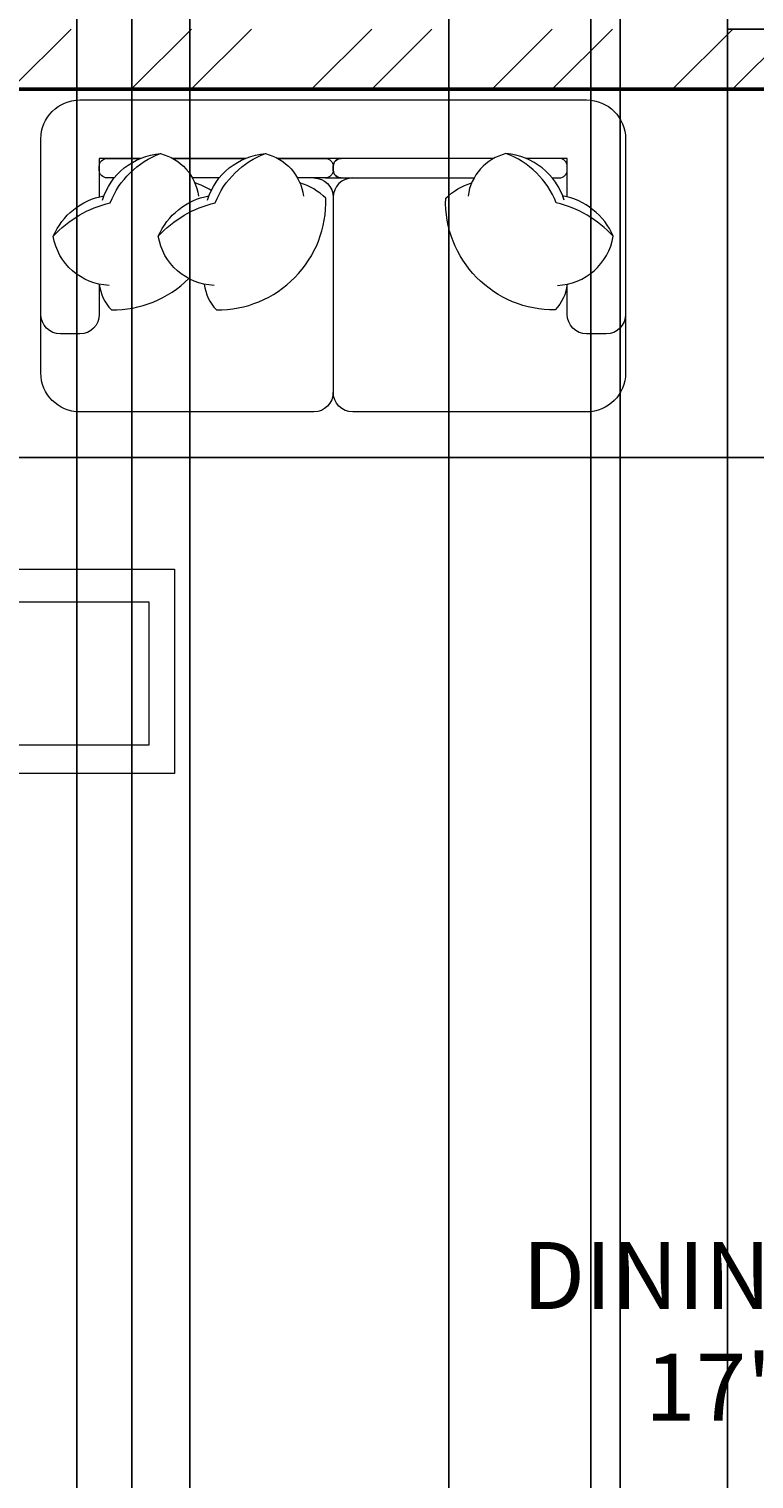
# Model space of a CAD drawing. Units: inches. Extents: x 2310 to 2937, y 1113 to 2410.
# Tile 6 of 23: x 2472 to 2526, y 1891 to 2000. Entities that reach past the tile are written whole.
import ezdxf

# ---------------------------------------------------------------- set-up
doc = ezdxf.new("R2010")
doc.units = ezdxf.units.IN
for name, color, linetype, lineweight in [('A-ANNO-DIMS', 2, 'Continuous', 18), ('A-AREA-IDEN', 7, 'Continuous', 18), ('A-FURN', 8, 'Continuous', 18), ('A-WALL', 7, 'Continuous', 50), ('A-WALL-PATT', 85, 'Continuous', 13)]:
    doc.layers.add(name, color=color, linetype=linetype, lineweight=lineweight)
doc.styles.get("Standard").update_dxf_attribs({"font": 'arial.ttf'})
doc.dimstyles.get("Standard").update_dxf_attribs({"dimtxt": 0.18, "dimasz": 0.18, "dimexe": 0.18, "dimexo": 0.0625, "dimgap": 0.09, "dimtad": 0, "dimtih": 1, "dimtoh": 1, "dimdec": 4, "dimzin": 0, "dimdsep": 46, "dimtxsty": 'Standard', "dimcen": 0.09, "dimadec": 0, "dimazin": 0, "dimtfac": 1, "dimtdec": 4, "dimtofl": 0, "dimtmove": 0, "dimatfit": 3, "dimfxl": 1, "dimtolj": 1, "dimtzin": 0, "dimarcsym": 0})

# ---------------------------------------------------------------- blocks, each defined once
blk = doc.blocks.new('*D41')
at = {"layer": 'A-ANNO-DIMS', "color": 0, "lineweight": -2, "transparency": 16777216}
for p, q in [((2479.99, 2347.45), (2479.99, 1649.5)), ((2503.66, 2347.45), (2503.66, 1649.5)), ((2480.17, 1649.68), (2491.36, 1649.68)), ((2503.48, 1649.68), (2492.29, 1649.68))]:
    blk.add_line(p, q, dxfattribs=at)
at = {"layer": 'A-ANNO-DIMS', "color": 0, "transparency": 16777216}
for points in [[(2480.17, 1649.71), (2480.17, 1649.65), (2479.99, 1649.68)], [(2503.48, 1649.71), (2503.48, 1649.65), (2503.66, 1649.68)]]:
    blk.add_solid(points, dxfattribs=at)
at = {"layer": 'Defpoints', "color": 0, "transparency": 16777216}
for p in [(2479.99, 2347.51), (2503.66, 2347.51), (2503.66, 1649.68)]:
    blk.add_point(p, dxfattribs=at)
at = {"layer": 'A-ANNO-DIMS', "color": 0, "transparency": 16777216, "insert": (2491.82, 1649.68), "char_height": 0.18, "attachment_point": 5}
blk.add_mtext('\\A1;23.676', dxfattribs=at)
blk = doc.blocks.new('*D57')
at = {"layer": 'A-ANNO-DIMS', "color": 0, "lineweight": -2, "transparency": 16777216}
for p, q in [((2403.55, 1995.01), (2858.02, 1995.01)), ((2857.84, 1994.83), (2857.84, 1981.45)), ((2857.84, 1967.7), (2857.84, 1981.09)), ((2403.55, 1967.52), (2858.02, 1967.52))]:
    blk.add_line(p, q, dxfattribs=at)
at = {"layer": 'A-ANNO-DIMS', "color": 0, "transparency": 16777216}
for points in [[(2857.81, 1994.83), (2857.87, 1994.83), (2857.84, 1995.01)], [(2857.81, 1967.7), (2857.87, 1967.7), (2857.84, 1967.52)]]:
    blk.add_solid(points, dxfattribs=at)
at = {"layer": 'Defpoints', "color": 0, "transparency": 16777216}
for p in [(2403.49, 1995.01), (2403.49, 1967.52), (2857.84, 1967.52)]:
    blk.add_point(p, dxfattribs=at)
at = {"layer": 'A-ANNO-DIMS', "color": 0, "transparency": 16777216, "insert": (2857.84, 1981.27), "char_height": 0.18, "attachment_point": 5}
blk.add_mtext('\\A1;27.49', dxfattribs=at)
blk = doc.blocks.new('*D61')
at = {"layer": 'A-ANNO-DIMS', "color": 0, "lineweight": -2, "transparency": 16777216}
for p, q in [((2484.33, 2205.95), (2484.33, 1649.5)), ((2514.27, 2205.95), (2514.27, 1649.5)), ((2484.51, 1649.68), (2498.9, 1649.68)), ((2514.09, 1649.68), (2499.69, 1649.68))]:
    blk.add_line(p, q, dxfattribs=at)
at = {"layer": 'A-ANNO-DIMS', "color": 0, "transparency": 16777216}
for points in [[(2484.51, 1649.71), (2484.51, 1649.65), (2484.33, 1649.68)], [(2514.09, 1649.71), (2514.09, 1649.65), (2514.27, 1649.68)]]:
    blk.add_solid(points, dxfattribs=at)
at = {"layer": 'Defpoints', "color": 0, "transparency": 16777216}
for p in [(2484.33, 2206.01), (2514.27, 2206.01), (2514.27, 1649.68)]:
    blk.add_point(p, dxfattribs=at)
at = {"layer": 'A-ANNO-DIMS', "color": 0, "transparency": 16777216, "insert": (2499.3, 1649.68), "char_height": 0.18, "attachment_point": 5}
blk.add_mtext('\\A1;29.94', dxfattribs=at)
blk = doc.blocks.new('*D63')
at = {"layer": 'A-ANNO-DIMS', "color": 0, "lineweight": -2, "transparency": 16777216}
for p, q in [((2436.46, 1999.45), (2436.46, 1649.5)), ((2524.46, 1999.45), (2524.46, 1649.5)), ((2436.64, 1649.68), (2480.25, 1649.68)), ((2524.28, 1649.68), (2480.68, 1649.68))]:
    blk.add_line(p, q, dxfattribs=at)
at = {"layer": 'A-ANNO-DIMS', "color": 0, "transparency": 16777216}
for points in [[(2436.64, 1649.71), (2436.64, 1649.65), (2436.46, 1649.68)], [(2524.28, 1649.71), (2524.28, 1649.65), (2524.46, 1649.68)]]:
    blk.add_solid(points, dxfattribs=at)
at = {"layer": 'Defpoints', "color": 0, "transparency": 16777216}
for p in [(2436.46, 1999.51), (2524.46, 1999.51), (2524.46, 1649.68)]:
    blk.add_point(p, dxfattribs=at)
at = {"layer": 'A-ANNO-DIMS', "color": 0, "transparency": 16777216, "insert": (2480.46, 1649.68), "char_height": 0.18, "attachment_point": 5}
blk.add_mtext('\\A1;88', dxfattribs=at)
blk = doc.blocks.new('*D64')
at = {"layer": 'A-ANNO-DIMS', "color": 0, "lineweight": -2, "transparency": 16777216}
for p, q in [((2524.527191, 2046.513944), (2858.015941, 2046.513944)), ((2857.835941, 2046.333944), (2857.835941, 2023.193944)), ((2857.835941, 1999.693944), (2857.835941, 2022.833944)), ((2524.527191, 1999.513944), (2858.015941, 1999.513944))]:
    blk.add_line(p, q, dxfattribs=at)
at = {"layer": 'A-ANNO-DIMS', "color": 0, "transparency": 16777216}
for points in [[(2857.805941, 2046.333944), (2857.865941, 2046.333944), (2857.835941, 2046.513944)], [(2857.805941, 1999.693944), (2857.865941, 1999.693944), (2857.835941, 1999.513944)]]:
    blk.add_solid(points, dxfattribs=at)
at = {"layer": 'Defpoints', "color": 0, "transparency": 16777216}
for p in [(2524.464691, 2046.513944), (2857.835941, 2046.513944), (2524.464691, 1999.513944)]:
    blk.add_point(p, dxfattribs=at)
at = {"layer": 'A-ANNO-DIMS', "color": 0, "transparency": 16777216, "insert": (2857.835941, 2023.013944), "char_height": 0.18, "attachment_point": 5}
blk.add_mtext('\\A1;47', dxfattribs=at)
blk = doc.blocks.new('*D66')
at = {"layer": 'A-ANNO-DIMS', "color": 0, "lineweight": -2, "transparency": 16777216}
for p, q in [((2516.46, 2093.45), (2516.46, 1649.5)), ((2524.46, 2093.45), (2524.46, 1649.5)), ((2516.64, 1649.68), (2520.32, 1649.68)), ((2524.28, 1649.68), (2520.61, 1649.68))]:
    blk.add_line(p, q, dxfattribs=at)
at = {"layer": 'A-ANNO-DIMS', "color": 0, "transparency": 16777216}
for points in [[(2516.64, 1649.71), (2516.64, 1649.65), (2516.46, 1649.68)], [(2524.28, 1649.71), (2524.28, 1649.65), (2524.46, 1649.68)]]:
    blk.add_solid(points, dxfattribs=at)
at = {"layer": 'Defpoints', "color": 0, "transparency": 16777216}
for p in [(2516.46, 2093.51), (2524.46, 2093.51), (2524.46, 1649.68)]:
    blk.add_point(p, dxfattribs=at)
at = {"layer": 'A-ANNO-DIMS', "color": 0, "transparency": 16777216, "insert": (2520.46, 1649.68), "char_height": 0.18, "attachment_point": 5}
blk.add_mtext('\\A1;8', dxfattribs=at)
blk = doc.blocks.new('*D69')
at = {"layer": 'A-ANNO-DIMS', "color": 0, "lineweight": -2, "transparency": 16777216}
for p, q in [((2441.86, 2131.96), (2441.86, 1649.5)), ((2475.89, 2131.96), (2475.89, 1649.5)), ((2442.04, 1649.68), (2458.48, 1649.68)), ((2475.71, 1649.68), (2459.27, 1649.68))]:
    blk.add_line(p, q, dxfattribs=at)
at = {"layer": 'A-ANNO-DIMS', "color": 0, "transparency": 16777216}
for points in [[(2442.04, 1649.71), (2442.04, 1649.65), (2441.86, 1649.68)], [(2475.71, 1649.71), (2475.71, 1649.65), (2475.89, 1649.68)]]:
    blk.add_solid(points, dxfattribs=at)
at = {"layer": 'Defpoints', "color": 0, "transparency": 16777216}
for p in [(2441.86, 2132.02), (2475.89, 2132.02), (2475.89, 1649.68)]:
    blk.add_point(p, dxfattribs=at)
at = {"layer": 'A-ANNO-DIMS', "color": 0, "transparency": 16777216, "insert": (2458.88, 1649.68), "char_height": 0.18, "attachment_point": 5}
blk.add_mtext('\\A1;34.03', dxfattribs=at)

msp = doc.modelspace()

# ---------------------------------------------------------------- hatches: boundary and pattern name
at = {"layer": 'A-WALL-PATT'}
h = msp.add_hatch(dxfattribs=at)
h.set_pattern_fill('ANSI32', color=256)
h.paths.add_polyline_path([(2639.1394, 2356.5139), (2563.662, 2356.5139), (2563.662, 2347.5139), (2606.9859, 2347.5139), (2606.9859, 2210.5139), (2514.2692, 2210.5139), (2514.2692, 2206.0139), (2606.9859, 2206.0139), (2606.9859, 2098.0139), (2602.689, 2098.0139), (2602.689, 2093.5139), (2615.5262, 2093.5139), (2615.5262, 2095.7639), (2615.5262, 2098.0139), (2611.4859, 2098.0139), (2611.4859, 2206.0139), (2703.9391, 2206.0139), (2703.9391, 2208.2639), (2703.9391, 2210.5139), (2611.4859, 2210.5139), (2611.4859, 2347.5139), (2639.1394, 2347.5139)])
h.paths.add_polyline_path([(2823.9859, 2356.5139), (2699.1394, 2356.5139), (2699.1394, 2347.5139), (2738.4859, 2347.5139), (2738.4859, 2343.9266), (2742.9859, 2343.9266), (2742.9859, 2347.5139), (2814.9859, 2347.5139), (2814.9859, 2336.76), (2823.9859, 2336.76)])
h.paths.add_polyline_path([(2823.9859, 2312.76), (2814.9859, 2312.76), (2814.9859, 2299.5139), (2742.9859, 2299.5139), (2742.9859, 2323.0159), (2740.7359, 2323.0159), (2738.4859, 2323.0159), (2738.4859, 2210.5139), (2734.5483, 2210.5139), (2734.5483, 2206.0139), (2746.8769, 2206.0139), (2746.8769, 2208.2639), (2746.8769, 2210.5139), (2742.9859, 2210.5139), (2742.9859, 2295.0139), (2814.9859, 2295.0139), (2814.9859, 2269.8977), (2823.9859, 2269.8977)])
h.paths.add_polyline_path([(2823.9859, 2210.5139), (2823.9859, 2233.8977), (2819.4859, 2233.8977), (2814.9859, 2233.8977), (2814.9859, 2210.5139), (2769.9745, 2210.5139), (2769.9745, 2206.0139), (2814.9859, 2206.0139), (2814.9859, 2178.3027), (2823.9859, 2178.3027)])
h.paths.add_polyline_path([(2823.9859, 2118.3027), (2819.4859, 2118.3027), (2814.9859, 2118.3027), (2814.9859, 2098.0139), (2647.0333, 2098.0139), (2647.0333, 2093.5139), (2814.9859, 2093.5139), (2814.9859, 1999.5139), (2650.6052, 1999.5139), (2650.6052, 1995.0139), (2814.9859, 1995.0139), (2814.9859, 1969.9784), (2823.9859, 1969.9784)])
h.paths.add_polyline_path([(2403.4859, 2093.5139), (2569.9888, 2093.5139), (2569.9888, 2095.7639), (2569.9888, 2098.0139), (2403.4859, 2098.0139), (2403.4859, 2131.7587), (2394.4859, 2131.7587), (2394.4859, 1967.522), (2403.4859, 1967.522), (2403.4859, 1995.0139), (2569.8903, 1995.0139), (2569.8903, 1997.2639), (2569.8903, 1999.5139), (2403.4859, 1999.5139)])
h.paths.add_polyline_path([(2503.662, 2356.5139), (2394.4859, 2356.5139), (2394.4859, 2337.9231), (2398.9859, 2337.9231), (2403.4859, 2337.9231), (2403.4859, 2347.5139), (2475.4859, 2347.5139), (2475.4859, 2343.0384), (2479.9859, 2343.0384), (2479.9859, 2347.5139), (2503.662, 2347.5139)])
h.paths.add_polyline_path([(2498.3065, 1745.5139), (2479.9859, 1745.5139), (2479.9859, 1749.1663), (2477.7359, 1749.1663), (2475.4859, 1749.1663), (2475.4859, 1745.5139), (2403.4859, 1745.5139), (2403.4859, 1753.6409), (2398.9859, 1753.6409), (2394.4859, 1753.6409), (2394.4859, 1736.5139), (2498.3065, 1736.5139), (2498.3065, 1741.0139)])
h.paths.add_polyline_path([(2479.9859, 1882.5139), (2483.9367, 1882.5139), (2483.9367, 1887.0139), (2471.5501, 1887.0139), (2471.5501, 1885.1969), (2471.5501, 1882.5139), (2475.4859, 1882.5139), (2475.4859, 1798.0139), (2403.4859, 1798.0139), (2403.4859, 1828.0433), (2402.2852, 1828.0433), (2394.4859, 1828.0433), (2394.4859, 1777.6409), (2403.4859, 1777.6409), (2403.4859, 1793.5139), (2475.4859, 1793.5139), (2475.4859, 1769.1696), (2479.9859, 1769.1696)])
h.paths.add_polyline_path([(2403.4859, 1907.522), (2398.9859, 1907.522), (2394.4859, 1907.522), (2394.4859, 1864.0433), (2403.4859, 1864.0433), (2403.4859, 1882.5139), (2448.9325, 1882.5139), (2448.9325, 1884.7639), (2448.9325, 1887.0139), (2403.4859, 1887.0139)])
h.paths.add_polyline_path([(2702.2061, 1887.0139), (2611.4859, 1887.0139), (2611.4859, 1995.0139), (2615.6132, 1995.0139), (2615.6132, 1999.5139), (2602.4798, 1999.5139), (2602.4798, 1997.2639), (2602.4798, 1995.0139), (2606.9859, 1995.0139), (2606.9859, 1887.0139), (2516.2443, 1887.0139), (2516.2443, 1884.7639), (2516.2443, 1882.5139), (2606.9859, 1882.5139), (2606.9859, 1745.5139), (2558.3065, 1745.5139), (2558.3065, 1736.5139), (2638.8921, 1736.5139), (2638.8921, 1741.0139), (2638.8921, 1745.5139), (2611.4859, 1745.5139), (2611.4859, 1882.5139), (2702.2061, 1882.5139)])
h.paths.add_polyline_path([(2823.9859, 1909.9784), (2819.4859, 1909.9784), (2814.9859, 1909.9784), (2814.9859, 1887.0139), (2769.144, 1887.0139), (2769.144, 1884.7639), (2769.144, 1882.5139), (2814.9859, 1882.5139), (2814.9859, 1854.1704), (2823.9859, 1854.1704)])
h.paths.add_polyline_path([(2823.9859, 1818.1704), (2819.4859, 1818.1704), (2814.9859, 1818.1704), (2814.9859, 1798.0139), (2742.9859, 1798.0139), (2742.9859, 1882.5139), (2746.805, 1882.5139), (2746.805, 1887.0139), (2733.7334, 1887.0139), (2733.7334, 1884.7639), (2733.7334, 1882.5139), (2738.4859, 1882.5139), (2738.4859, 1771.1728), (2740.7359, 1771.1728), (2742.9859, 1771.1728), (2742.9859, 1793.5139), (2814.9859, 1793.5139), (2814.9859, 1783.6684), (2823.9859, 1783.6684)])
h.paths.add_polyline_path([(2823.9859, 1759.6684), (2814.9859, 1759.6684), (2814.9859, 1745.5139), (2742.9859, 1745.5139), (2742.9859, 1748.9831), (2740.7359, 1748.9831), (2738.4859, 1748.9831), (2738.4859, 1745.5139), (2698.8921, 1745.5139), (2698.8921, 1736.5139), (2823.9859, 1736.5139)])

# ---------------------------------------------------------------- linework, layer by layer
at = {"layer": 'A-FURN', "ltscale": 0.03}
msp.add_lwpolyline([(2496.4919, 1970.9338, -0.41421356), (2495.0368, 1972.389, -0.41421356), (2493.5816, 1970.9338), (2476.1193, 1970.9338, -0.41421356), (2473.2089, 1973.8442), (2473.2089, 1991.3064, -0.41421356), (2476.1193, 1994.2168), (2513.9542, 1994.2168, -0.41421356), (2516.8646, 1991.3064), (2516.8646, 1973.8442, -0.41421356), (2513.9542, 1970.9338), (2496.4919, 1970.9338, -0.41421356), (2495.0368, 1972.389, -0.41421356), (2493.5816, 1970.9338)], format="xyb", dxfattribs=at)
at = {"layer": 'A-FURN'}
for points in [[(2474.1351, 1984.0442, -0.14772988), (2478.3882, 1986.5451, -0.21334276), (2482.1409, 1990.2131, -0.17866181)], [(2480.6358, 1989.8512), (2477.5745, 1989.8512), (2477.5745, 1986.9914, -0.41421356)], [(2478.685, 1988.396), (2478.1566, 1988.396, -0.41421356), (2477.5745, 1988.9781), (2477.5745, 1989.2692, -0.41421356), (2478.1566, 1989.8512)], [(2477.8006, 1986.7444, -0.30666349), (2482.1409, 1990.2131, -0.30632997), (2484.9763, 1987.0453, 0.87284716)], [(2478.1566, 1989.8512), (2480.6358, 1989.8512, -0.41421356)], [(2481.9741, 1984.0442, -0.14772988), (2486.2272, 1986.5451, -0.21334276), (2489.9799, 1990.2131, -0.17866181)], [(2483.0567, 1989.8512), (2488.4748, 1989.8512, -0.41421356)], [(2485.6396, 1986.7444, -0.30666349), (2489.9799, 1990.2131, -0.30632997), (2492.8153, 1987.0453, 0.87284716)], [(2490.8958, 1989.8512), (2494.4547, 1989.8512, -0.41421356), (2495.0368, 1989.2692), (2495.0368, 1988.9781, -0.41421356), (2494.4547, 1988.396), (2492.361, 1988.396, -0.41421356)], [(2507.0168, 1989.8512), (2495.6188, 1989.8512, 0.41421356), (2495.0368, 1989.2692), (2495.0368, 1988.9781, 0.41421356), (2495.6188, 1988.396), (2505.5515, 1988.396, 0.41421356)], [(2512.2729, 1986.7444, 0.30666349), (2507.9326, 1990.2131, 0.30632997), (2505.0972, 1987.0453, -0.87284716)], [(2515.9385, 1984.0442, 0.14772988), (2511.6854, 1986.5451, 0.21334276), (2507.9326, 1990.2131, 0.17866181)], [(2511.9169, 1989.8512), (2509.4377, 1989.8512, 0.41421356)], [(2511.3885, 1988.396), (2511.9169, 1988.396, 0.41421356), (2512.499, 1988.9781), (2512.499, 1989.2692, 0.41421356), (2511.9169, 1989.8512)], [(2486.524, 1988.396), (2484.522, 1988.396, -0.41421356)], [(2493.5816, 1988.396, -0.41421356), (2495.0368, 1986.9409)], [(2493.5816, 1988.396, -0.41421356), (2495.0368, 1986.9409), (2495.0368, 1972.389, -0.41421356)], [(2496.4919, 1988.396, 0.41421356), (2495.0368, 1986.9409)], [(2496.4919, 1988.396, 0.41421356), (2495.0368, 1986.9409), (2495.0368, 1972.389, 0.41421356)], [(2485.9242, 1987.4587, 0.07186538), (2484.7041, 1988.0276, -7.11546429)], [(2485.4104, 1980.465, 0.16554063), (2486.3106, 1978.5423, 0.42598917), (2494.4832, 1986.8786, 0.12152332), (2492.5432, 1988.0276, -7.11546429)], [(2512.5022, 1980.465, -0.16554063), (2511.602, 1978.5423, -0.42598917), (2503.4293, 1986.8786, -0.12152332), (2505.3694, 1988.0276, 7.11546429)], [(2478.3048, 1980.3763, -0.35677236), (2474.1351, 1984.0442, -0.24954205), (2477.9132, 1987.067, 9.61688035)], [(2486.1438, 1980.3763, -0.35677236), (2481.9741, 1984.0442, -0.24954205), (2485.7522, 1987.067, 9.61688035)], [(2511.7687, 1980.3763, 0.35677236), (2515.9385, 1984.0442, 0.24954205), (2512.1603, 1987.067, -9.61688035)], [(2477.5713, 1980.465, 0.16554063), (2478.4715, 1978.5423, 0.20023115), (2484.2481, 1980.884, 0.12152332)], [(2477.5745, 1980.4643), (2477.5745, 1978.2097, -0.41421356), (2476.1193, 1976.7545), (2474.6641, 1976.7545, -0.41421356), (2473.2089, 1978.2097)], [(2516.8646, 1978.2097, -0.41421356), (2515.4094, 1976.7545), (2513.9542, 1976.7545, -0.41421356), (2512.499, 1978.2097), (2512.499, 1980.4643)]]:
    msp.add_lwpolyline(points, format="xyb", dxfattribs=at)
for points in [[(2488.4748, 1989.8512), (2483.0567, 1989.8512)], [(2507.0168, 1989.8512), (2490.8958, 1989.8512)], [(2512.499, 1986.9914), (2512.499, 1989.8512), (2509.4377, 1989.8512)]]:
    msp.add_lwpolyline(points, dxfattribs=at)
msp.add_lwpolyline([(2495.6188, 1989.8512), (2494.4547, 1989.8512, -0.41421356), (2495.0368, 1989.2692), (2495.0368, 1988.9781, -0.41421356), (2494.4547, 1988.396), (2495.6188, 1988.396, -0.41421356), (2495.0368, 1988.9781), (2495.0368, 1989.2692, -0.41421356)], format="xyb", close=True, dxfattribs=at)
for points in [[(2449.1475, 1959.1855), (2483.1791, 1959.1855), (2483.1791, 1943.9281), (2449.1475, 1943.9281)], [(2450.9745, 1956.7439), (2481.2801, 1956.7439), (2481.2801, 1946.0624), (2450.9745, 1946.0624)]]:
    msp.add_lwpolyline(points, close=True, dxfattribs=at)
at = {"layer": 'A-WALL'}
msp.add_line((2403.4859, 1995.0139), (2571.4589, 1995.0139), dxfattribs=at)

# ---------------------------------------------------------------- texts
at = {"layer": 'A-AREA-IDEN', "insert": (2495.3926, 1908.9628), "char_height": 5, "attachment_point": 1}
msp.add_mtext_dynamic_manual_height_columns("         DINING CUM LIVING\\P               17'X9'", width=186.629206, gutter_width=12.5, heights=[0], dxfattribs=at)

# ---------------------------------------------------------------- dimensions: what is measured, and where the dimension line sits
at = {"layer": 'A-ANNO-DIMS'}
for base, p1, p2, override, picture, middle in [((2503.662, 1649.6807), (2479.9859, 2347.5139), (2503.662, 2347.5139), {"dimdec": 3, "dimlfac": 1, "dimrnd": 0, "dimzin": 0, "dimdsep": 46, "dimlunit": 2}, '*D41', (2491.824, 1649.6807)), ((2514.2692, 1649.6807), (2484.3278, 2206.0139), (2514.2692, 2206.0139), {"dimdec": 2, "dimlfac": 1, "dimrnd": 0, "dimzin": 0, "dimdsep": 46, "dimlunit": 2}, '*D61', (2499.2985, 1649.6807)), ((2475.8929, 1649.6807), (2441.8613, 2132.0241), (2475.8929, 2132.0241), {"dimdec": 2, "dimlfac": 1, "dimrnd": 0, "dimzin": 0, "dimdsep": 46, "dimlunit": 2}, '*D69', (2458.8771, 1649.6807)), ((2524.4647, 1649.6807), (2516.4647, 2093.5139), (2524.4647, 2093.5139), {"dimdec": 0, "dimlfac": 1, "dimrnd": 0, "dimzin": 0, "dimdsep": 46, "dimlunit": 2}, '*D66', (2520.4647, 1649.6807)), ((2524.4647, 1649.6807), (2436.4647, 1999.5139), (2524.4647, 1999.5139), {"dimdec": 0, "dimlfac": 1, "dimrnd": 0, "dimzin": 0, "dimdsep": 46, "dimlunit": 2}, '*D63', (2480.4647, 1649.6807))]:
    dim = msp.add_linear_dim(base=base, p1=p1, p2=p2, dimstyle='Standard', override=override, dxfattribs=at)
    dim.commit()
    dim.dimension.update_dxf_attribs({"geometry": picture, "text_midpoint": middle})
for base, p1, p2, override, picture, middle in [((2857.8359, 2046.5139), (2524.4647, 1999.5139), (2524.4647, 2046.5139), {"dimdec": 0, "dimlfac": 1, "dimrnd": 0, "dimzin": 0, "dimdsep": 46, "dimlunit": 2}, '*D64', (2857.8359, 2023.0139)), ((2857.8359, 1967.522), (2403.4859, 1995.0139), (2403.4859, 1967.522), {"dimdec": 2, "dimlfac": 1, "dimrnd": 0, "dimzin": 0, "dimdsep": 46, "dimlunit": 2}, '*D57', (2857.8359, 1981.268))]:
    dim = msp.add_linear_dim(base=base, p1=p1, p2=p2, angle=90, dimstyle='Standard', override=override, dxfattribs=at)
    dim.commit()
    dim.dimension.update_dxf_attribs({"geometry": picture, "text_midpoint": middle})

doc.saveas('drawing.dxf')
